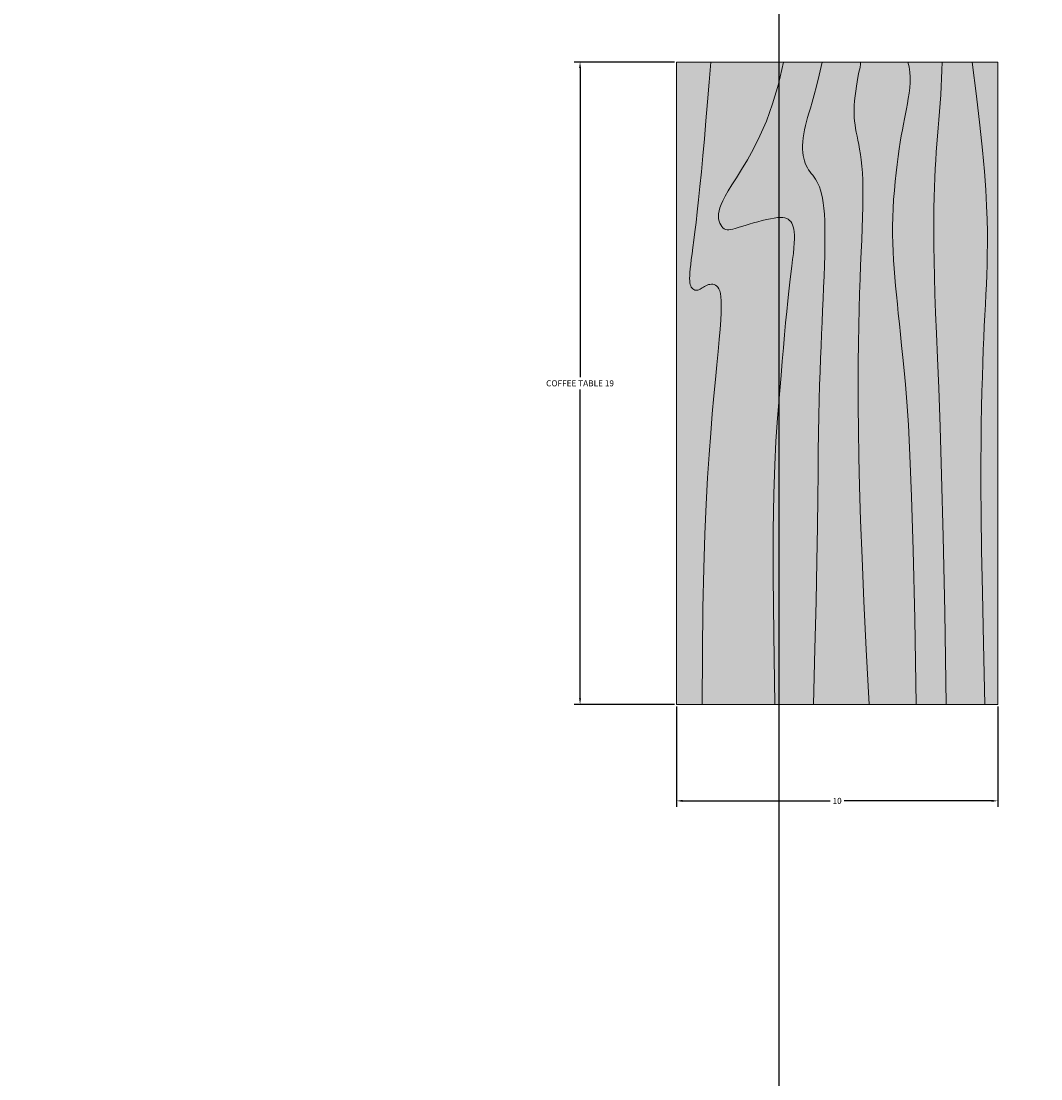
# Model space of a CAD drawing. Units: inches. Extents: x 857 to 1111, y 424 to 822.
# Tile 6 of 9: x 1031 to 1062, y 636 to 668. Entities that reach past the tile are written whole.
import ezdxf

# ---------------------------------------------------------------- set-up
doc = ezdxf.new("R2010")
doc.units = ezdxf.units.IN
for name, color, linetype, lineweight in [('A-ANNO-DIMS', 2, 'Continuous', 18), ('A-FURN', 8, 'Continuous', 18), ('A-FURN-PATT', 9, 'Continuous', 13)]:
    doc.layers.add(name, color=color, linetype=linetype, lineweight=lineweight)
doc.styles.get("Standard").update_dxf_attribs({"font": 'arial.ttf'})
doc.dimstyles.get("Standard").update_dxf_attribs({"dimtxt": 0.18, "dimasz": 0.18, "dimexe": 0.18, "dimexo": 0.0625, "dimgap": 0.09, "dimtad": 0, "dimtih": 1, "dimtoh": 1, "dimdec": 4, "dimzin": 0, "dimdsep": 46, "dimtxsty": 'Standard', "dimcen": 0.09, "dimadec": 0, "dimazin": 0, "dimtfac": 1, "dimtdec": 4, "dimtofl": 0, "dimtmove": 0, "dimatfit": 3, "dimfxl": 1, "dimtolj": 1, "dimtzin": 0, "dimarcsym": 0})

# ---------------------------------------------------------------- blocks, each defined once
blk = doc.blocks.new('Table - Rectangular Woodgrain 60 x 30 in.')
for p, q in [((0, 0), (0, -30)), ((60, 0), (0, 0)), ((60, -30), (60, 0)), ((0, -30), (60, -30))]:
    blk.add_line(p, q)
for points in [[(0, -2.4), (4.8155, -2.418), (9.0302, -2.4688), (12.709, -2.5477), (15.9167, -2.65), (18.7181, -2.7711), (21.1781, -2.9063), (23.3616, -3.0508), (25.3333, -3.2), (27.1477, -3.3495), (28.8172, -3.4958), (30.3437, -3.636), (31.7291, -3.7667), (32.9756, -3.8849), (34.0849, -3.9875), (35.059, -4.0714), (35.9, -4.1334), (36.6114, -4.1711), (37.2041, -4.1854), (37.6906, -4.1779), (38.0833, -4.15), (38.3948, -4.1034), (38.6375, -4.0396), (38.8239, -3.9602), (38.9666, -3.8667), (39.0764, -3.7608), (39.1573, -3.6448), (39.2116, -3.521), (39.2416, -3.3917), (39.2498, -3.2593), (39.2385, -3.1261), (39.21, -2.9944), (39.1666, -2.8667), (39.111, -2.7447), (39.0468, -2.6281), (38.978, -2.5163), (38.9083, -2.4083), (38.8418, -2.3035), (38.7823, -2.201), (38.7337, -2.1001), (38.7, -2), (38.6844, -1.9003), (38.6875, -1.8021), (38.7094, -1.707), (38.75, -1.6167), (38.8094, -1.5326), (38.8875, -1.4563), (38.9844, -1.3893), (39.1, -1.3333), (39.2351, -1.2896), (39.3937, -1.2583), (39.5804, -1.2396), (39.8, -1.2333), (40.057, -1.2396), (40.3562, -1.2583), (40.7023, -1.2896), (41.1, -1.3333), (41.5547, -1.3895), (42.0755, -1.4573), (42.6721, -1.5361), (43.3542, -1.625), (44.1316, -1.7233), (45.014, -1.8302), (46.0114, -1.9449), (47.1333, -2.0667), (48.3862, -2.1947), (49.7625, -2.3281), (51.2513, -2.4663), (52.8416, -2.6083), (54.5226, -2.7535), (56.2833, -2.9011), (58.1127, -3.0501), (60, -3.2)], [(0, -9.2), (6.5759, -9.0858), (11.9385, -9.0365), (16.2527, -9.0418), (19.6833, -9.0917), (22.3952, -9.1759), (24.5531, -9.2844), (26.322, -9.4069), (27.8666, -9.5333), (29.3241, -9.6553), (30.7203, -9.7719), (32.0532, -9.8837), (33.3208, -9.9917), (34.5213, -10.0965), (35.6526, -10.199), (36.7128, -10.2999), (37.7, -10.4), (38.6129, -10.4996), (39.4531, -10.5969), (40.223, -10.6895), (40.925, -10.775), (41.5613, -10.8512), (42.1344, -10.9156), (42.6465, -10.966), (43.1, -11), (43.4976, -11.0158), (43.8437, -11.0136), (44.143, -10.9942), (44.4, -10.9583), (44.6195, -10.9069), (44.8062, -10.8406), (44.9648, -10.7603), (45.1, -10.6667), (45.2155, -10.5598), (45.3114, -10.4365), (45.3871, -10.2929), (45.4416, -10.125), (45.4743, -9.929), (45.4844, -9.7011), (45.4709, -9.4371), (45.4333, -9.1333), (45.3716, -8.7883), (45.2896, -8.4104), (45.1919, -8.0107), (45.0833, -7.6), (44.9685, -7.1893), (44.8521, -6.7896), (44.7388, -6.4117), (44.6333, -6.0667), (44.54, -5.7628), (44.4614, -5.4979), (44.4001, -5.2675), (44.3583, -5.0667), (44.3384, -4.8909), (44.3427, -4.7354), (44.3736, -4.5956), (44.4333, -4.4667), (44.5236, -4.3453), (44.6427, -4.2333), (44.7884, -4.1339), (44.9583, -4.05), (45.1501, -3.9849), (45.3614, -3.9417), (45.59, -3.9234), (45.8333, -3.9333), (46.0915, -3.9749), (46.3734, -4.0531), (46.6906, -4.1736), (47.0542, -4.3417), (47.4756, -4.5629), (47.9661, -4.8427), (48.5372, -5.1866), (49.2, -5.6), (49.9676, -6.0844), (50.8594, -6.625), (51.8965, -7.2031), (53.1, -7.8), (54.491, -8.3969), (56.0906, -8.975), (57.9199, -9.5156), (60, -10)], [(0, -12.8), (5.1847, -12.9322), (9.6213, -13.0323), (13.3963, -13.1059), (16.5958, -13.1583), (19.3063, -13.1952), (21.614, -13.2219), (23.6054, -13.2439), (25.3666, -13.2667), (26.9728, -13.2947), (28.4531, -13.3281), (29.8256, -13.3663), (31.1083, -13.4083), (32.3191, -13.4535), (33.476, -13.501), (34.597, -13.5501), (35.7, -13.6), (36.7984, -13.6497), (37.8875, -13.6979), (38.9578, -13.743), (40, -13.7833), (41.0047, -13.8174), (41.9625, -13.8438), (42.864, -13.8607), (43.7, -13.8667), (44.4631, -13.8604), (45.1552, -13.8417), (45.7801, -13.8104), (46.3416, -13.7667), (46.8439, -13.7104), (47.2906, -13.6417), (47.6858, -13.5604), (48.0333, -13.4667), (48.3375, -13.3608), (48.6042, -13.2448), (48.8396, -13.121), (49.05, -12.9917), (49.2417, -12.8593), (49.4208, -12.7261), (49.5937, -12.5944), (49.7667, -12.4667), (49.9452, -12.3451), (50.1323, -12.2313), (50.3303, -12.1268), (50.5416, -12.0333), (50.7686, -11.9524), (51.0135, -11.8854), (51.2788, -11.8341), (51.5666, -11.8), (51.8785, -11.7843), (52.2116, -11.7865), (52.562, -11.8059), (52.926, -11.8417), (53.2998, -11.8931), (53.6795, -11.9594), (54.0614, -12.0397), (54.4416, -12.1333), (54.8223, -12.2401), (55.2293, -12.3625), (55.6942, -12.5037), (56.2489, -12.6667), (56.9251, -12.8547), (57.7545, -13.0708), (58.7689, -13.3182), (60, -13.6)], [(0, -18), (5.124, -17.7273), (9.6609, -17.5057), (13.6705, -17.3303), (17.2125, -17.1958), (20.3467, -17.0973), (23.1328, -17.0297), (25.6307, -16.9878), (27.9, -16.9667), (29.9928, -16.9617), (31.9302, -16.9703), (33.7254, -16.9907), (35.3917, -17.0208), (36.9423, -17.0588), (38.3906, -17.1026), (39.7499, -17.1503), (41.0333, -17.2), (42.2519, -17.2496), (43.4073, -17.2969), (44.4986, -17.3395), (45.525, -17.375), (46.4858, -17.4012), (47.3802, -17.4156), (48.2074, -17.416), (48.9667, -17.4), (49.6583, -17.3662), (50.2872, -17.3167), (50.8595, -17.2547), (51.3812, -17.1833), (51.8584, -17.1057), (52.2971, -17.025), (52.7034, -16.9443), (53.0833, -16.8667), (53.443, -16.7951), (53.789, -16.7313), (54.128, -16.6768), (54.4666, -16.6334), (54.8115, -16.6024), (55.1693, -16.5854), (55.5465, -16.5841), (55.95, -16.6), (56.3828, -16.6337), (56.8346, -16.6823), (57.2915, -16.7418), (57.7396, -16.8084), (58.165, -16.878), (58.5539, -16.9469), (58.8924, -17.0111), (59.1666, -17.0667), (59.3679, -17.1107), (59.5078, -17.1438), (59.6032, -17.1675), (59.6708, -17.1833), (59.7275, -17.193), (59.7901, -17.1979), (59.8753, -17.1998), (60, -17.2)], [(0, -22.4), (8.0098, -22.2501), (14.4094, -22.1011), (19.4168, -21.9535), (23.25, -21.8083), (26.1269, -21.6663), (28.2656, -21.5281), (29.884, -21.3947), (31.2, -21.2667), (32.3967, -21.1448), (33.5172, -21.0292), (34.5697, -20.9198), (35.5625, -20.8167), (36.5037, -20.7198), (37.4015, -20.6292), (38.2642, -20.5448), (39.1, -20.4667), (39.9164, -20.3951), (40.7187, -20.3313), (41.5117, -20.2768), (42.3, -20.2333), (43.0883, -20.2024), (43.8812, -20.1854), (44.6836, -20.1841), (45.5, -20.2), (46.3328, -20.234), (47.1747, -20.2844), (48.0163, -20.3488), (48.8479, -20.425), (49.66, -20.5106), (50.4429, -20.6031), (51.1872, -20.7004), (51.8833, -20.8), (52.5246, -20.8999), (53.1166, -20.9995), (53.6681, -21.0983), (54.1875, -21.1958), (54.6834, -21.2919), (55.1646, -21.3859), (55.6394, -21.4777), (56.1167, -21.5667), (56.6028, -21.6515), (57.0961, -21.7266), (57.5929, -21.7852), (58.0896, -21.8208), (58.5823, -21.8268), (59.0674, -21.7964), (59.5412, -21.723), (60, -21.6)], [(0, -25.2), (8.6355, -25.0504), (15.7026, -24.9031), (21.4049, -24.7606), (25.9458, -24.625), (29.529, -24.4988), (32.3578, -24.3844), (34.6359, -24.284), (36.5667, -24.2), (38.3213, -24.1341), (39.9417, -24.0854), (41.437, -24.0523), (42.8167, -24.0333), (44.0901, -24.0268), (45.2667, -24.0313), (46.3557, -24.0451), (47.3667, -24.0667), (48.309, -24.0947), (49.1928, -24.1287), (50.0284, -24.168), (50.826, -24.2125), (51.5959, -24.2617), (52.3483, -24.3151), (53.0935, -24.3725), (53.8417, -24.4334), (54.6009, -24.497), (55.3699, -24.561), (56.1454, -24.6226), (56.9239, -24.6792), (57.7021, -24.7279), (58.4764, -24.7662), (59.2435, -24.7911), (60, -24.8)], [(0, -28.8), (5.6867, -28.6681), (10.45, -28.5698), (14.407, -28.5012), (17.675, -28.4584), (20.3711, -28.4374), (22.6125, -28.4344), (24.5164, -28.4455), (26.2, -28.4667), (27.762, -28.4947), (29.2276, -28.5281), (30.6033, -28.5663), (31.8958, -28.6084), (33.1118, -28.6535), (34.2578, -28.7011), (35.3405, -28.7501), (36.3666, -28.8), (37.3443, -28.8497), (38.288, -28.8974), (39.2137, -28.9412), (40.1375, -28.9792), (41.0753, -29.0093), (42.0432, -29.0297), (43.0572, -29.0384), (44.1333, -29.0333), (45.2936, -29.0114), (46.5843, -28.9641), (48.0579, -28.8816), (49.7666, -28.7542), (51.7629, -28.5721), (54.0989, -28.3255), (56.8272, -28.0048), (60, -27.6)]]:
    blk.add_lwpolyline(points)
blk = doc.blocks.new('*D32')
at = {"layer": 'A-ANNO-DIMS', "color": 0, "lineweight": -2, "transparency": 16777216}
for p, q in [((1050.864, 666.568), (1047.878, 666.568)), ((1048.058, 666.388), (1048.058, 657.19)), ((1048.058, 647.626), (1048.058, 656.824)), ((1050.864, 647.446), (1047.878, 647.446))]:
    blk.add_line(p, q, dxfattribs=at)
at = {"layer": 'A-ANNO-DIMS', "color": 0, "transparency": 16777216}
for points in [[(1048.028, 666.388), (1048.088, 666.388), (1048.058, 666.568)], [(1048.028, 647.626), (1048.088, 647.626), (1048.058, 647.446)]]:
    blk.add_solid(points, dxfattribs=at)
at = {"layer": 'Defpoints', "color": 0, "transparency": 16777216}
for p in [(1048.058, 666.568), (1050.927, 666.568), (1050.927, 647.446)]:
    blk.add_point(p, dxfattribs=at)
at = {"layer": 'A-ANNO-DIMS', "color": 0, "transparency": 16777216, "insert": (1048.058, 657.007), "char_height": 0.18, "attachment_point": 5}
blk.add_mtext('\\A1;COFFEE TABLE 19', dxfattribs=at)
blk = doc.blocks.new('*D33')
at = {"layer": 'A-ANNO-DIMS', "color": 0, "lineweight": -2, "transparency": 16777216}
for p, q in [((1050.927, 647.383), (1050.927, 644.397)), ((1060.488, 647.383), (1060.488, 644.397)), ((1051.107, 644.577), (1055.497, 644.577)), ((1060.308, 644.577), (1055.918, 644.577))]:
    blk.add_line(p, q, dxfattribs=at)
at = {"layer": 'A-ANNO-DIMS', "color": 0, "transparency": 16777216}
for points in [[(1051.107, 644.607), (1051.107, 644.547), (1050.927, 644.577)], [(1060.308, 644.607), (1060.308, 644.547), (1060.488, 644.577)]]:
    blk.add_solid(points, dxfattribs=at)
at = {"layer": 'Defpoints', "color": 0, "transparency": 16777216}
for p in [(1050.927, 647.446), (1060.488, 647.446), (1050.927, 644.577)]:
    blk.add_point(p, dxfattribs=at)
at = {"layer": 'A-ANNO-DIMS', "color": 0, "transparency": 16777216, "insert": (1055.708, 644.577), "char_height": 0.18, "attachment_point": 5}
blk.add_mtext('\\A1;10', dxfattribs=at)
blk = doc.blocks.new('*D55')
at = {"layer": 'A-ANNO-DIMS', "color": 0, "lineweight": -2, "transparency": 16777216}
for p, q in [((1053.972, 717.294), (1053.972, 423.627)), ((1083.137, 717.294), (1083.137, 423.627)), ((1054.152, 423.807), (1068.088, 423.807)), ((1082.957, 423.807), (1069.02, 423.807))]:
    blk.add_line(p, q, dxfattribs=at)
at = {"layer": 'A-ANNO-DIMS', "color": 0, "transparency": 16777216}
for points in [[(1054.152, 423.837), (1054.152, 423.777), (1053.972, 423.807)], [(1082.957, 423.837), (1082.957, 423.777), (1083.137, 423.807)]]:
    blk.add_solid(points, dxfattribs=at)
at = {"layer": 'Defpoints', "color": 0, "transparency": 16777216}
for p in [(1053.972, 717.357), (1083.137, 717.357), (1083.137, 423.807)]:
    blk.add_point(p, dxfattribs=at)
at = {"layer": 'A-ANNO-DIMS', "color": 0, "transparency": 16777216, "insert": (1068.554, 423.807), "char_height": 0.18, "attachment_point": 5}
blk.add_mtext('\\A1;29.165', dxfattribs=at)
blk = doc.blocks.new('*D56')
at = {"layer": 'A-ANNO-DIMS', "color": 0, "lineweight": -2, "transparency": 16777216}
for p, q in [((924.77, 717.294), (924.77, 423.627)), ((1053.972, 717.294), (1053.972, 423.627)), ((924.95, 423.807), (988.986, 423.807)), ((1053.792, 423.807), (989.755, 423.807))]:
    blk.add_line(p, q, dxfattribs=at)
at = {"layer": 'A-ANNO-DIMS', "color": 0, "transparency": 16777216}
for points in [[(924.95, 423.837), (924.95, 423.777), (924.77, 423.807)], [(1053.792, 423.837), (1053.792, 423.777), (1053.972, 423.807)]]:
    blk.add_solid(points, dxfattribs=at)
at = {"layer": 'Defpoints', "color": 0, "transparency": 16777216}
for p in [(924.77, 717.357), (1053.972, 717.357), (1053.972, 423.807)]:
    blk.add_point(p, dxfattribs=at)
at = {"layer": 'A-ANNO-DIMS', "color": 0, "transparency": 16777216, "insert": (989.371, 423.807), "char_height": 0.18, "attachment_point": 5}
blk.add_mtext('\\A1;129.2', dxfattribs=at)

msp = doc.modelspace()

# ---------------------------------------------------------------- hatches: boundary and pattern name
at = {"layer": 'A-FURN-PATT'}
h = msp.add_hatch(color=256, dxfattribs=at)
h.dxf.hatch_style = 1
h.paths.add_polyline_path([(1060.4882, 666.5682), (1059.7233, 666.5682), (1059.8523, 665.557), (1059.9545, 664.6875), (1060.0331, 663.943), (1060.0911, 663.3068), (1060.1317, 662.7622), (1060.158, 662.2925), (1060.1731, 661.8812), (1060.1801, 661.5114), (1060.1817, 661.1684), (1060.1789, 660.8452), (1060.1724, 660.5368), (1060.1628, 660.2379), (1060.1507, 659.9435), (1060.1367, 659.6484), (1060.1215, 659.3477), (1060.1057, 659.0361), (1060.0898, 658.709), (1060.0742, 658.364), (1060.059, 657.9987), (1060.0446, 657.6112), (1060.0312, 657.1992), (1060.019, 656.7608), (1060.0084, 656.2937), (1059.9995, 655.7959), (1059.9927, 655.2593), (1059.9892, 654.6525), (1059.9901, 653.9381), (1059.9968, 653.0789), (1060.0105, 652.0373), (1060.0323, 650.7762), (1060.0637, 649.2581), (1060.1057, 647.4457), (1060.4882, 647.4457)])
h.paths.add_polyline_path([(1060.019, 656.7608), (1060.0312, 657.1992), (1060.0446, 657.6112), (1060.059, 657.9987), (1060.0742, 658.364), (1060.0898, 658.709), (1060.1057, 659.0361), (1060.1215, 659.3477), (1060.1367, 659.6484), (1060.1507, 659.9435), (1060.1628, 660.2379), (1060.1724, 660.5368), (1060.1789, 660.8452), (1060.1817, 661.1684), (1060.1801, 661.5114), (1060.1731, 661.8812), (1060.158, 662.2925), (1060.1317, 662.7622), (1060.0911, 663.3068), (1060.0331, 663.943), (1059.9545, 664.6875), (1059.8523, 665.557), (1059.7233, 666.5682), (1058.8309, 666.5682), (1058.828, 666.3271), (1058.8201, 666.0827), (1058.8079, 665.8359), (1058.7924, 665.5879), (1058.7743, 665.3398), (1058.7547, 665.0926), (1058.7343, 664.8475), (1058.714, 664.6055), (1058.6946, 664.3671), (1058.6763, 664.1296), (1058.6593, 663.8898), (1058.6436, 663.6444), (1058.6294, 663.3902), (1058.6169, 663.1239), (1058.6061, 662.8422), (1058.5972, 662.5419), (1058.5903, 662.2197), (1058.5859, 661.8726), (1058.5844, 661.4976), (1058.5865, 661.0918), (1058.5926, 660.652), (1058.6031, 660.1755), (1058.6186, 659.659), (1058.6396, 659.0998), (1058.6664, 658.4845), (1058.6984, 657.7584), (1058.7349, 656.8568), (1058.7751, 655.7148), (1058.8183, 654.2676), (1058.8637, 652.4502), (1058.9107, 650.1979), (1058.9583, 647.4457), (1060.1057, 647.4457), (1060.0637, 649.2581), (1060.0323, 650.7762), (1060.0105, 652.0373), (1059.9968, 653.0789), (1059.9901, 653.9381), (1059.9892, 654.6525), (1059.9927, 655.2593), (1059.9995, 655.7959), (1060.0084, 656.2937)])
h.paths.add_polyline_path([(1058.6664, 658.4845), (1058.6396, 659.0998), (1058.6186, 659.659), (1058.6031, 660.1755), (1058.5926, 660.652), (1058.5865, 661.0918), (1058.5844, 661.4976), (1058.5859, 661.8726), (1058.5903, 662.2197), (1058.5972, 662.5419), (1058.6061, 662.8422), (1058.6169, 663.1239), (1058.6294, 663.3902), (1058.6436, 663.6444), (1058.6593, 663.8898), (1058.6763, 664.1296), (1058.6946, 664.3671), (1058.714, 664.6055), (1058.7343, 664.8475), (1058.7547, 665.0926), (1058.7743, 665.3398), (1058.7924, 665.5879), (1058.8079, 665.8359), (1058.8201, 666.0827), (1058.828, 666.3271), (1058.8309, 666.5682), (1057.811, 666.5682), (1057.8502, 666.422), (1057.8736, 666.271), (1057.8833, 666.1164), (1057.8814, 665.9594), (1057.87, 665.8011), (1057.8513, 665.6427), (1057.8274, 665.4855), (1057.8004, 665.3306), (1057.772, 665.1785), (1057.7428, 665.0272), (1057.7128, 664.8738), (1057.6822, 664.7157), (1057.6511, 664.5502), (1057.6196, 664.3744), (1057.5879, 664.1858), (1057.556, 663.9814), (1057.5243, 663.7595), (1057.4933, 663.5223), (1057.4638, 663.2728), (1057.4365, 663.014), (1057.4122, 662.7489), (1057.3917, 662.4807), (1057.3756, 662.2124), (1057.3648, 661.947), (1057.3597, 661.6868), (1057.3601, 661.431), (1057.3656, 661.1783), (1057.3754, 660.9271), (1057.3893, 660.6758), (1057.4066, 660.4231), (1057.427, 660.1674), (1057.4498, 659.9072), (1057.4747, 659.6408), (1057.5016, 659.3659), (1057.5305, 659.0798), (1057.5613, 658.7798), (1057.5942, 658.4634), (1057.6291, 658.1279), (1057.6659, 657.7708), (1057.7048, 657.3894), (1057.7456, 656.97), (1057.7881, 656.4542), (1057.8321, 655.7726), (1057.8774, 654.8557), (1057.9237, 653.634), (1057.9707, 652.0381), (1058.0182, 649.9985), (1058.066, 647.4457), (1058.9583, 647.4457), (1058.9107, 650.1979), (1058.8637, 652.4502), (1058.8183, 654.2676), (1058.7751, 655.7148), (1058.7349, 656.8568), (1058.6984, 657.7584)])
h.paths.add_polyline_path([(1057.6659, 657.7708), (1057.6291, 658.1279), (1057.5942, 658.4634), (1057.5613, 658.7798), (1057.5305, 659.0798), (1057.5016, 659.3659), (1057.4747, 659.6408), (1057.4498, 659.9072), (1057.427, 660.1674), (1057.4066, 660.4231), (1057.3893, 660.6758), (1057.3754, 660.9271), (1057.3656, 661.1783), (1057.3601, 661.431), (1057.3597, 661.6868), (1057.3648, 661.947), (1057.3756, 662.2124), (1057.3917, 662.4807), (1057.4122, 662.7489), (1057.4365, 663.014), (1057.4638, 663.2728), (1057.4933, 663.5223), (1057.5243, 663.7595), (1057.556, 663.9814), (1057.5879, 664.1858), (1057.6196, 664.3744), (1057.6511, 664.5502), (1057.6822, 664.7157), (1057.7128, 664.8738), (1057.7428, 665.0272), (1057.772, 665.1785), (1057.8004, 665.3306), (1057.8274, 665.4855), (1057.8513, 665.6427), (1057.87, 665.8011), (1057.8814, 665.9594), (1057.8833, 666.1164), (1057.8736, 666.271), (1057.8502, 666.422), (1057.811, 666.5682), (1056.4087, 666.5682), (1056.4086, 666.5087), (1056.4059, 666.4741), (1056.3983, 666.4418), (1056.3908, 666.4114), (1056.3802, 666.3668), (1056.3662, 666.3026), (1056.3485, 666.2152), (1056.328, 666.1074), (1056.306, 665.9834), (1056.2839, 665.8478), (1056.2626, 665.705), (1056.2437, 665.5594), (1056.2282, 665.4154), (1056.2174, 665.2775), (1056.2124, 665.1489), (1056.2128, 665.0287), (1056.2182, 664.9146), (1056.2281, 664.8047), (1056.2419, 664.6968), (1056.2593, 664.5887), (1056.2796, 664.4785), (1056.3024, 664.3638), (1056.3272, 664.2428), (1056.3529, 664.1133), (1056.3786, 663.9734), (1056.4033, 663.8214), (1056.4261, 663.6551), (1056.4459, 663.4727), (1056.4616, 663.2722), (1056.4724, 663.0518), (1056.4775, 662.8098), (1056.4774, 662.5462), (1056.4728, 662.2611), (1056.4644, 661.9549), (1056.4531, 661.6278), (1056.4396, 661.28), (1056.4245, 660.9118), (1056.4087, 660.5234), (1056.3928, 660.1143), (1056.3776, 659.6811), (1056.3637, 659.2195), (1056.3516, 658.7253), (1056.342, 658.1943), (1056.3355, 657.6221), (1056.3327, 657.0047), (1056.3343, 656.3377), (1056.341, 655.6144), (1056.3544, 654.8183), (1056.3759, 653.9304), (1056.4073, 652.9315), (1056.4502, 651.8026), (1056.5061, 650.5247), (1056.5767, 649.0787), (1056.6636, 647.4457), (1058.066, 647.4457), (1058.0182, 649.9985), (1057.9707, 652.0381), (1057.9237, 653.634), (1057.8774, 654.8557), (1057.8321, 655.7726), (1057.7881, 656.4542), (1057.7456, 656.97), (1057.7048, 657.3894)])
h.paths.add_polyline_path([(1056.3327, 657.0047), (1056.3355, 657.6221), (1056.342, 658.1943), (1056.3516, 658.7253), (1056.3637, 659.2195), (1056.3776, 659.6811), (1056.3928, 660.1143), (1056.4087, 660.5234), (1056.4245, 660.9118), (1056.4396, 661.28), (1056.4531, 661.6278), (1056.4644, 661.9549), (1056.4728, 662.2611), (1056.4774, 662.5462), (1056.4775, 662.8098), (1056.4724, 663.0518), (1056.4616, 663.2722), (1056.4459, 663.4727), (1056.4261, 663.6551), (1056.4033, 663.8214), (1056.3786, 663.9734), (1056.3529, 664.1133), (1056.3272, 664.2428), (1056.3024, 664.3638), (1056.2796, 664.4785), (1056.2593, 664.5887), (1056.2419, 664.6968), (1056.2281, 664.8047), (1056.2182, 664.9146), (1056.2128, 665.0287), (1056.2124, 665.1489), (1056.2174, 665.2775), (1056.2282, 665.4154), (1056.2437, 665.5594), (1056.2626, 665.705), (1056.2839, 665.8478), (1056.306, 665.9834), (1056.328, 666.1074), (1056.3485, 666.2152), (1056.3662, 666.3026), (1056.3802, 666.3668), (1056.3908, 666.4114), (1056.3983, 666.4418), (1056.4033, 666.4633), (1056.4064, 666.4814), (1056.408, 666.5014), (1056.4086, 666.5285), (1056.4087, 666.5682), (1055.2613, 666.5682), (1055.1715, 666.1759), (1055.0927, 665.8526), (1055.0238, 665.5882), (1054.9639, 665.3727), (1054.9119, 665.1959), (1054.8669, 665.0478), (1054.8279, 664.9181), (1054.7939, 664.7967), (1054.764, 664.6756), (1054.7384, 664.5538), (1054.7173, 664.4328), (1054.7009, 664.3137), (1054.6895, 664.1977), (1054.6833, 664.086), (1054.6826, 663.9798), (1054.6876, 663.8804), (1054.6985, 663.7887), (1054.7149, 663.7042), (1054.7362, 663.6261), (1054.762, 663.5538), (1054.7918, 663.4864), (1054.8251, 663.4233), (1054.8614, 663.3637), (1054.9001, 663.3068), (1054.9408, 663.2517), (1054.9828, 663.1966), (1055.0252, 663.1395), (1055.0674, 663.0784), (1055.1087, 663.0113), (1055.1481, 662.9363), (1055.1851, 662.8513), (1055.2188, 662.7543), (1055.2487, 662.6436), (1055.2746, 662.5176), (1055.2965, 662.3753), (1055.3144, 662.2152), (1055.3284, 662.0362), (1055.3383, 661.8371), (1055.3443, 661.6165), (1055.3463, 661.3733), (1055.3444, 661.1068), (1055.339, 660.8195), (1055.3306, 660.5143), (1055.3197, 660.1941), (1055.3069, 659.8619), (1055.2925, 659.5208), (1055.2772, 659.1737), (1055.2613, 658.8236), (1055.2454, 658.4721), (1055.2298, 658.1148), (1055.2146, 657.7461), (1055.2002, 657.3602), (1055.1868, 656.9514), (1055.1747, 656.5139), (1055.164, 656.0422), (1055.1551, 655.5303), (1055.1478, 654.9689), (1055.1408, 654.3343), (1055.1323, 653.5988), (1055.1205, 652.7349), (1055.1038, 651.7152), (1055.0804, 650.5121), (1055.0485, 649.0981), (1055.0063, 647.4457), (1056.6636, 647.4457), (1056.5767, 649.0787), (1056.5061, 650.5247), (1056.4502, 651.8026), (1056.4073, 652.9315), (1056.3759, 653.9304), (1056.3544, 654.8183), (1056.341, 655.6144), (1056.3343, 656.3377)])
h.paths.add_polyline_path([(1055.1408, 654.3343), (1055.1478, 654.9689), (1055.1551, 655.5303), (1055.164, 656.0422), (1055.1747, 656.5139), (1055.1868, 656.9514), (1055.2002, 657.3602), (1055.2146, 657.7461), (1055.2298, 658.1148), (1055.2454, 658.4721), (1055.2613, 658.8236), (1055.2772, 659.1737), (1055.2925, 659.5208), (1055.3069, 659.8619), (1055.3197, 660.1941), (1055.3306, 660.5143), (1055.339, 660.8195), (1055.3444, 661.1068), (1055.3463, 661.3733), (1055.3443, 661.6165), (1055.3383, 661.8371), (1055.3284, 662.0362), (1055.3144, 662.2152), (1055.2965, 662.3753), (1055.2746, 662.5176), (1055.2487, 662.6436), (1055.2188, 662.7543), (1055.1851, 662.8513), (1055.1481, 662.9363), (1055.1087, 663.0113), (1055.0674, 663.0784), (1055.0252, 663.1395), (1054.9828, 663.1966), (1054.9408, 663.2517), (1054.9001, 663.3068), (1054.8614, 663.3637), (1054.8251, 663.4233), (1054.7918, 663.4864), (1054.762, 663.5538), (1054.7362, 663.6261), (1054.7149, 663.7042), (1054.6985, 663.7887), (1054.6876, 663.8804), (1054.6826, 663.9798), (1054.6833, 664.086), (1054.6895, 664.1977), (1054.7009, 664.3137), (1054.7173, 664.4328), (1054.7384, 664.5538), (1054.764, 664.6756), (1054.7939, 664.7967), (1054.8279, 664.9181), (1054.8669, 665.0478), (1054.9119, 665.1959), (1054.9639, 665.3727), (1055.0238, 665.5882), (1055.0927, 665.8526), (1055.1715, 666.1759), (1055.2613, 666.5682), (1054.114, 666.5682), (1053.9596, 665.9053), (1053.7873, 665.3223), (1053.603, 664.8125), (1053.4128, 664.3692), (1053.2226, 663.9856), (1053.0383, 663.6551), (1052.866, 663.3708), (1052.7116, 663.1262), (1052.5799, 662.9149), (1052.4703, 662.7329), (1052.3811, 662.5766), (1052.3106, 662.4423), (1052.257, 662.3264), (1052.2186, 662.2253), (1052.1937, 662.1355), (1052.1804, 662.0532), (1052.1773, 661.9756), (1052.1831, 661.9028), (1052.1969, 661.8354), (1052.2176, 661.7743), (1052.2444, 661.7202), (1052.2761, 661.6737), (1052.3118, 661.6358), (1052.3504, 661.607), (1052.3915, 661.588), (1052.4361, 661.5781), (1052.4856, 661.5767), (1052.5417, 661.5831), (1052.6057, 661.5964), (1052.6791, 661.6159), (1052.7635, 661.641), (1052.8604, 661.6707), (1052.9703, 661.7044), (1053.0908, 661.7405), (1053.2182, 661.7776), (1053.3491, 661.8142), (1053.48, 661.8488), (1053.6073, 661.8799), (1053.7278, 661.906), (1053.8377, 661.9257), (1053.9346, 661.9377), (1054.0187, 661.942), (1054.0913, 661.9388), (1054.1538, 661.9283), (1054.2073, 661.911), (1054.2531, 661.8869), (1054.2924, 661.8563), (1054.3264, 661.8195), (1054.3563, 661.7764), (1054.3819, 661.7258), (1054.403, 661.6663), (1054.4194, 661.5964), (1054.4308, 661.5145), (1054.437, 661.4191), (1054.4377, 661.3088), (1054.4327, 661.1821), (1054.4218, 661.0375), (1054.4058, 660.8743), (1054.3852, 660.6917), (1054.361, 660.4889), (1054.3337, 660.2651), (1054.3042, 660.0198), (1054.2732, 659.752), (1054.2414, 659.461), (1054.2095, 659.1464), (1054.1774, 658.8085), (1054.1447, 658.4479), (1054.1113, 658.0653), (1054.0769, 657.6613), (1054.0413, 657.2365), (1054.0041, 656.7915), (1053.9652, 656.327), (1053.9249, 655.8347), (1053.8859, 655.271), (1053.8513, 654.5832), (1053.8245, 653.7189), (1053.8086, 652.6256), (1053.8069, 651.2506), (1053.8226, 649.5415), (1053.859, 647.4457), (1055.0063, 647.4457), (1055.0485, 649.0981), (1055.0804, 650.5121), (1055.1038, 651.7152), (1055.1205, 652.7349), (1055.1323, 653.5988)])
h.paths.add_polyline_path([(1053.8513, 654.5832), (1053.8859, 655.271), (1053.9249, 655.8347), (1053.9652, 656.327), (1054.0041, 656.7915), (1054.0413, 657.2365), (1054.0769, 657.6613), (1054.1113, 658.0653), (1054.1447, 658.4479), (1054.1774, 658.8085), (1054.2095, 659.1464), (1054.2414, 659.461), (1054.2732, 659.752), (1054.3042, 660.0198), (1054.3337, 660.2651), (1054.361, 660.4889), (1054.3852, 660.6917), (1054.4058, 660.8743), (1054.4218, 661.0375), (1054.4327, 661.1821), (1054.4377, 661.3088), (1054.437, 661.4191), (1054.4308, 661.5145), (1054.4194, 661.5964), (1054.403, 661.6663), (1054.3819, 661.7258), (1054.3563, 661.7764), (1054.3264, 661.8195), (1054.2924, 661.8563), (1054.2531, 661.8869), (1054.2073, 661.911), (1054.1538, 661.9283), (1054.0913, 661.9388), (1054.0187, 661.942), (1053.9346, 661.9377), (1053.8377, 661.9257), (1053.7278, 661.906), (1053.6073, 661.8799), (1053.48, 661.8488), (1053.3491, 661.8142), (1053.2182, 661.7776), (1053.0908, 661.7405), (1052.9703, 661.7044), (1052.8604, 661.6707), (1052.7635, 661.641), (1052.6791, 661.6159), (1052.6057, 661.5964), (1052.5417, 661.5831), (1052.4856, 661.5767), (1052.4361, 661.5781), (1052.3915, 661.588), (1052.3504, 661.607), (1052.3118, 661.6358), (1052.2761, 661.6737), (1052.2444, 661.7202), (1052.2176, 661.7743), (1052.1969, 661.8354), (1052.1831, 661.9028), (1052.1773, 661.9756), (1052.1804, 662.0532), (1052.1937, 662.1355), (1052.2186, 662.2253), (1052.257, 662.3264), (1052.3106, 662.4423), (1052.3811, 662.5766), (1052.4703, 662.7329), (1052.5799, 662.9149), (1052.7116, 663.1262), (1052.866, 663.3708), (1053.0383, 663.6551), (1053.2226, 663.9856), (1053.4128, 664.3692), (1053.603, 664.8125), (1053.7873, 665.3223), (1053.9596, 665.9053), (1054.114, 666.5682), (1051.9467, 666.5682), (1051.899, 665.9667), (1051.8515, 665.3837), (1051.8044, 664.8225), (1051.7582, 664.2868), (1051.7129, 663.78), (1051.6689, 663.3055), (1051.6263, 662.8668), (1051.5855, 662.4675), (1051.5467, 662.1099), (1051.5102, 661.7921), (1051.4761, 661.5108), (1051.4448, 661.2631), (1051.4164, 661.0457), (1051.3913, 660.8555), (1051.3697, 660.6896), (1051.3518, 660.5446), (1051.3379, 660.4179), (1051.3279, 660.3076), (1051.3219, 660.2122), (1051.3199, 660.1303), (1051.3219, 660.0603), (1051.3279, 660.0008), (1051.3379, 659.9503), (1051.3518, 659.9072), (1051.3696, 659.8704), (1051.391, 659.8395), (1051.4153, 659.8146), (1051.4421, 659.7957), (1051.4709, 659.7827), (1051.5012, 659.7757), (1051.5325, 659.7748), (1051.5643, 659.7797), (1051.5962, 659.7905), (1051.6283, 659.806), (1051.661, 659.8249), (1051.6944, 659.8461), (1051.7532, 659.8841), (1051.8016, 659.9107), (1051.8405, 659.9284), (1051.8812, 659.9423), (1051.9232, 659.9514), (1051.9656, 659.955), (1052.0078, 659.9523), (1052.049, 659.9428), (1052.0885, 659.9255), (1052.1255, 659.8997), (1052.1592, 659.8647), (1052.189, 659.8192), (1052.2143, 659.7598), (1052.2347, 659.6825), (1052.2495, 659.5832), (1052.2584, 659.458), (1052.2608, 659.303), (1052.2562, 659.1141), (1052.2442, 658.8873), (1052.2245, 658.6193), (1052.1977, 658.3089), (1052.165, 657.9553), (1052.1273, 657.558), (1052.0857, 657.1165), (1052.041, 656.63), (1051.9944, 656.0979), (1051.9467, 655.5196), (1051.8992, 654.8912), (1051.8531, 654.1953), (1051.81, 653.4113), (1051.7714, 652.5185), (1051.7388, 651.4962), (1051.7137, 650.3237), (1051.6975, 648.9804), (1051.6918, 647.4457), (1053.859, 647.4457), (1053.8226, 649.5415), (1053.8069, 651.2506), (1053.8086, 652.6256), (1053.8245, 653.7189)])
h.paths.add_polyline_path([(1052.0857, 657.1165), (1052.1273, 657.558), (1052.165, 657.9553), (1052.1977, 658.3089), (1052.2245, 658.6193), (1052.2442, 658.8873), (1052.2562, 659.1141), (1052.2608, 659.303), (1052.2584, 659.458), (1052.2495, 659.5832), (1052.2347, 659.6825), (1052.2143, 659.7598), (1052.189, 659.8192), (1052.1592, 659.8647), (1052.1255, 659.8997), (1052.0885, 659.9255), (1052.049, 659.9428), (1052.0078, 659.9523), (1051.9656, 659.955), (1051.9232, 659.9514), (1051.8812, 659.9423), (1051.8405, 659.9284), (1051.8016, 659.9107), (1051.7645, 659.8903), (1051.7288, 659.8683), (1051.6666, 659.8282), (1051.6092, 659.7949), (1051.5481, 659.7743), (1051.4853, 659.7763), (1051.4421, 659.7957), (1051.4153, 659.8146), (1051.391, 659.8395), (1051.3696, 659.8704), (1051.3518, 659.9072), (1051.3379, 659.9503), (1051.3279, 660.0008), (1051.3219, 660.0603), (1051.3199, 660.1303), (1051.3219, 660.2122), (1051.3279, 660.3076), (1051.3379, 660.4179), (1051.3518, 660.5446), (1051.3697, 660.6896), (1051.3913, 660.8555), (1051.4164, 661.0457), (1051.4448, 661.2631), (1051.4761, 661.5108), (1051.5102, 661.7921), (1051.5467, 662.1099), (1051.5855, 662.4675), (1051.6263, 662.8668), (1051.6689, 663.3055), (1051.7129, 663.78), (1051.7582, 664.2868), (1051.8044, 664.8225), (1051.8515, 665.3837), (1051.899, 665.9667), (1051.9467, 666.5682), (1050.9269, 666.5682), (1050.9269, 647.4457), (1051.6918, 647.4457), (1051.6975, 648.9804), (1051.7137, 650.3237), (1051.7388, 651.4962), (1051.7714, 652.5185), (1051.81, 653.4113), (1051.8531, 654.1953), (1051.8992, 654.8912), (1051.9467, 655.5196), (1051.9944, 656.0979), (1052.041, 656.63)])

# ---------------------------------------------------------------- block references
at = {"layer": 'A-FURN', "xscale": 0.3187096548202369, "yscale": 0.3187096548202369, "zscale": 0.3187096548202369, "rotation": 90}
msp.add_blockref('Table - Rectangular Woodgrain 60 x 30 in.', (1050.9269, 647.4457), dxfattribs=at)

# ---------------------------------------------------------------- dimensions: what is measured, and where the dimension line sits
at = {"layer": 'A-ANNO-DIMS'}
for base, p1, p2, override, picture, middle in [((1053.9717, 423.8067), (924.7696, 717.3567), (1053.9717, 717.3567), {"dimdec": 1, "dimlfac": 1, "dimrnd": 0, "dimzin": 0, "dimdsep": 46, "dimlunit": 2}, '*D56', (989.3707, 423.8067)), ((1083.1369, 423.8067), (1053.9717, 717.3567), (1083.1369, 717.3567), {"dimdec": 3, "dimlfac": 1, "dimrnd": 0, "dimzin": 0, "dimdsep": 46, "dimlunit": 2}, '*D55', (1068.5543, 423.8067))]:
    dim = msp.add_linear_dim(base=base, p1=p1, p2=p2, dimstyle='Standard', override=override, dxfattribs=at)
    dim.commit()
    dim.dimension.update_dxf_attribs({"geometry": picture, "text_midpoint": middle})
dim = msp.add_linear_dim(base=(1048.0585, 666.5682), p1=(1050.9269, 647.4457), p2=(1050.9269, 666.5682), angle=90, text='COFFEE TABLE <>', dimstyle='Standard', override={"dimdec": 0, "dimlfac": 1, "dimrnd": 0, "dimzin": 0, "dimdsep": 46, "dimlunit": 2}, dxfattribs=at)
dim.commit()
dim.dimension.update_dxf_attribs({"geometry": '*D32', "text_midpoint": (1048.0585, 657.007)})
dim = msp.add_linear_dim(base=(1050.9269, 644.5773), p1=(1060.4882, 647.4457), p2=(1050.9269, 647.4457), angle=180, dimstyle='Standard', override={"dimdec": 0, "dimlfac": 1, "dimrnd": 0, "dimzin": 0, "dimdsep": 46, "dimlunit": 2}, dxfattribs=at)
dim.commit()
dim.dimension.update_dxf_attribs({"geometry": '*D33', "text_midpoint": (1055.7075, 644.5773)})

doc.saveas('drawing.dxf')
